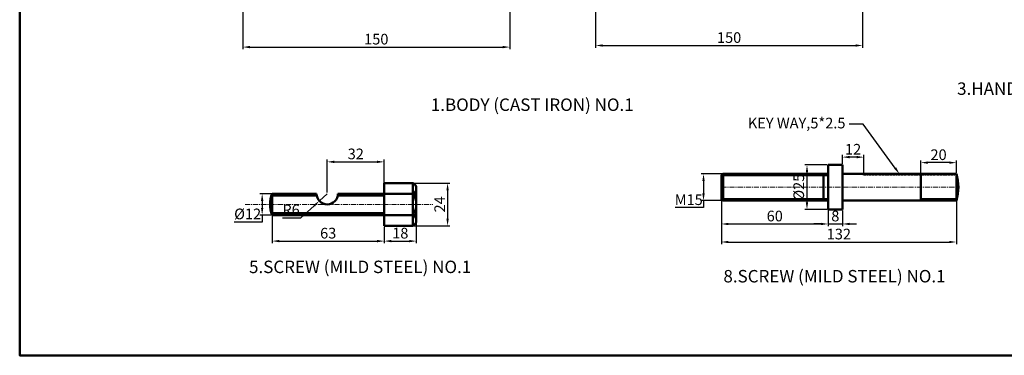
# Model space of a CAD drawing. Units: millimetres. Extents: x 177 to 1064, y 105 to 671.
# Tile 1 of 4: x 177 to 730, y 105 to 294. Entities that reach past the tile are written whole.
import ezdxf
from ezdxf import colors
from ezdxf.entities.mleader import LeaderData, LeaderLine
from ezdxf.math import Vec2, Vec3

# ---------------------------------------------------------------- set-up
doc = ezdxf.new("R2010")
doc.units = ezdxf.units.MM
doc.header["$LTSCALE"] = 0.3
doc.linetypes.add('CENTER', pattern=[50.8, 31.75, -6.35, 6.35, -6.35])
doc.linetypes.add('HIDDEN', pattern=[9.525, 6.35, -3.175])
for name, color, linetype, lineweight in [('M-CNTR', 1, 'CENTER', 18), ('M-DIMS', 2, 'Continuous', 25), ('M-HIDN', 6, 'HIDDEN', 25), ('M-OUTL', 7, 'Continuous', 50), ('M-TEXT', 3, 'Continuous', 25)]:
    doc.layers.add(name, color=color, linetype=linetype, lineweight=lineweight)
doc.styles.get("Standard").update_dxf_attribs({"font": 'arial.ttf'})
doc.dimstyles.new('ISO-25', dxfattribs={"dimtxt": 6, "dimasz": 4, "dimexe": 1.25, "dimexo": 0.625, "dimtad": 1, "dimtoh": 1, "dimtxsty": 'Standard', "dimcen": 2.5, "dimadec": 0, "dimazin": 0, "dimtfac": 1, "dimtmove": 0, "dimatfit": 3, "dimfxl": 1, "dimarcsym": 0})

# ---------------------------------------------------------------- blocks, each defined once
blk = doc.blocks.new('*D1')
at = {"layer": 'Defpoints', "color": 0, "ltscale": 0.2, "transparency": 16777216}
for p in [(302.04, 325.34), (452.04, 325.34), (452.04, 278.47)]:
    blk.add_point(p, dxfattribs=at)
at = {"layer": 'M-DIMS', "color": 0, "lineweight": -2, "ltscale": 0.2, "transparency": 16777216}
for p, q in [((302.04, 324.72), (302.04, 277.22)), ((452.04, 324.72), (452.04, 277.22)), ((306.04, 278.47), (448.04, 278.47))]:
    blk.add_line(p, q, dxfattribs=at)
at = {"layer": 'M-DIMS', "color": 0, "ltscale": 0.2, "transparency": 16777216}
for points in [[(306.04, 279.14), (306.04, 277.81), (302.04, 278.47)], [(448.04, 279.14), (448.04, 277.81), (452.04, 278.47)]]:
    blk.add_solid(points, dxfattribs=at)
at = {"layer": 'M-DIMS', "color": 0, "ltscale": 0.2, "transparency": 16777216, "insert": (377.04, 282.16), "char_height": 6, "attachment_point": 5}
blk.add_mtext('150', dxfattribs=at)
blk = doc.blocks.new('*D17')
at = {"layer": 'Defpoints', "color": 0, "ltscale": 0.2, "transparency": 16777216}
for p in [(500.2, 315.34), (650.2, 315.34), (650.2, 279.36)]:
    blk.add_point(p, dxfattribs=at)
at = {"layer": 'M-DIMS', "color": 0, "lineweight": -2, "ltscale": 0.2, "transparency": 16777216}
for p, q in [((500.2, 314.72), (500.2, 278.11)), ((650.2, 314.72), (650.2, 278.11)), ((504.2, 279.36), (646.2, 279.36))]:
    blk.add_line(p, q, dxfattribs=at)
at = {"layer": 'M-DIMS', "color": 0, "ltscale": 0.2, "transparency": 16777216}
for points in [[(504.2, 280.03), (504.2, 278.7), (500.2, 279.36)], [(646.2, 280.03), (646.2, 278.7), (650.2, 279.36)]]:
    blk.add_solid(points, dxfattribs=at)
at = {"layer": 'M-DIMS', "color": 0, "ltscale": 0.2, "transparency": 16777216, "insert": (575.2, 283.05), "char_height": 6, "attachment_point": 5}
blk.add_mtext('150', dxfattribs=at)
blk = doc.blocks.new('*D33')
at = {"layer": 'Defpoints', "color": 0, "ltscale": 0.3, "transparency": 16777216}
for p in [(381.52, 213.92), (349.52, 196), (381.52, 196)]:
    blk.add_point(p, dxfattribs=at)
at = {"layer": 'M-DIMS', "color": 0, "lineweight": -2, "ltscale": 0.3, "transparency": 16777216}
for p, q in [((349.52, 196.63), (349.52, 215.17)), ((353.52, 213.92), (377.52, 213.92)), ((381.52, 196.63), (381.52, 215.17))]:
    blk.add_line(p, q, dxfattribs=at)
at = {"layer": 'M-DIMS', "color": 0, "ltscale": 0.3, "transparency": 16777216}
for points in [[(353.52, 214.59), (353.52, 213.25), (349.52, 213.92)], [(377.52, 214.59), (377.52, 213.25), (381.52, 213.92)]]:
    blk.add_solid(points, dxfattribs=at)
at = {"layer": 'M-DIMS', "color": 0, "ltscale": 0.3, "transparency": 16777216, "insert": (365.52, 217.61), "char_height": 6, "attachment_point": 5}
blk.add_mtext('32', dxfattribs=at)
blk = doc.blocks.new('*D34')
at = {"layer": 'Defpoints', "color": 0, "ltscale": 0.3, "transparency": 16777216}
for p in [(318.52, 184), (381.52, 178), (381.52, 169.36)]:
    blk.add_point(p, dxfattribs=at)
at = {"layer": 'M-DIMS', "color": 0, "lineweight": -2, "ltscale": 0.3, "transparency": 16777216}
for p, q in [((318.52, 183.38), (318.52, 168.11)), ((381.52, 177.38), (381.52, 168.11)), ((322.52, 169.36), (377.52, 169.36))]:
    blk.add_line(p, q, dxfattribs=at)
at = {"layer": 'M-DIMS', "color": 0, "ltscale": 0.3, "transparency": 16777216}
for points in [[(322.52, 170.03), (322.52, 168.69), (318.52, 169.36)], [(377.52, 170.03), (377.52, 168.69), (381.52, 169.36)]]:
    blk.add_solid(points, dxfattribs=at)
at = {"layer": 'M-DIMS', "color": 0, "ltscale": 0.3, "transparency": 16777216, "insert": (350.02, 173.05), "char_height": 6, "attachment_point": 5}
blk.add_mtext('63', dxfattribs=at)
blk = doc.blocks.new('*D35')
at = {"layer": 'Defpoints', "color": 0, "ltscale": 0.3, "transparency": 16777216}
for p in [(331.02, 196), (312.94, 184), (331.02, 184)]:
    blk.add_point(p, dxfattribs=at)
at = {"layer": 'M-DIMS', "color": 0, "lineweight": -2, "ltscale": 0.3, "transparency": 16777216}
for p, q in [((330.4, 196), (311.69, 196)), ((312.94, 192), (312.94, 188)), ((330.4, 184), (311.69, 184)), ((312.94, 184), (312.94, 180)), ((312.94, 180), (297.26, 180))]:
    blk.add_line(p, q, dxfattribs=at)
at = {"layer": 'M-DIMS', "color": 0, "ltscale": 0.3, "transparency": 16777216}
for points in [[(312.28, 192), (313.61, 192), (312.94, 196)], [(312.28, 188), (313.61, 188), (312.94, 184)]]:
    blk.add_solid(points, dxfattribs=at)
at = {"layer": 'M-DIMS', "color": 0, "ltscale": 0.3, "transparency": 16777216, "insert": (304.79, 183.86), "char_height": 6, "attachment_point": 5}
blk.add_mtext('%%C12', dxfattribs=at)
blk = doc.blocks.new('*D36')
at = {"layer": 'Defpoints', "color": 0, "ltscale": 0.3, "transparency": 16777216}
for p in [(399.52, 184), (381.52, 178), (399.52, 169.36)]:
    blk.add_point(p, dxfattribs=at)
at = {"layer": 'M-DIMS', "color": 0, "lineweight": -2, "ltscale": 0.3, "transparency": 16777216}
for p, q in [((399.52, 183.38), (399.52, 168.11)), ((381.52, 177.38), (381.52, 168.11)), ((385.52, 169.36), (395.52, 169.36))]:
    blk.add_line(p, q, dxfattribs=at)
at = {"layer": 'M-DIMS', "color": 0, "ltscale": 0.3, "transparency": 16777216}
for points in [[(385.52, 170.03), (385.52, 168.69), (381.52, 169.36)], [(395.52, 170.03), (395.52, 168.69), (399.52, 169.36)]]:
    blk.add_solid(points, dxfattribs=at)
at = {"layer": 'M-DIMS', "color": 0, "ltscale": 0.3, "transparency": 16777216, "insert": (390.52, 173.05), "char_height": 6, "attachment_point": 5}
blk.add_mtext('18', dxfattribs=at)
blk = doc.blocks.new('*D37')
at = {"layer": 'Defpoints', "color": 0, "ltscale": 0.3, "transparency": 16777216}
for p in [(570.84, 199.67), (630.84, 199.67), (630.84, 178.99)]:
    blk.add_point(p, dxfattribs=at)
at = {"layer": 'M-DIMS', "color": 0, "lineweight": -2, "ltscale": 0.3, "transparency": 16777216}
for p, q in [((570.84, 199.04), (570.84, 177.74)), ((630.84, 199.04), (630.84, 177.74)), ((574.84, 178.99), (626.84, 178.99))]:
    blk.add_line(p, q, dxfattribs=at)
at = {"layer": 'M-DIMS', "color": 0, "ltscale": 0.3, "transparency": 16777216}
for points in [[(574.84, 179.65), (574.84, 178.32), (570.84, 178.99)], [(626.84, 179.65), (626.84, 178.32), (630.84, 178.99)]]:
    blk.add_solid(points, dxfattribs=at)
at = {"layer": 'M-DIMS', "color": 0, "ltscale": 0.3, "transparency": 16777216, "insert": (600.84, 182.67), "char_height": 6, "attachment_point": 5}
blk.add_mtext('60', dxfattribs=at)
blk = doc.blocks.new('*D38')
at = {"layer": 'Defpoints', "color": 0, "ltscale": 0.3, "transparency": 16777216}
for p in [(578.45, 207.17), (560.82, 192.17), (578.45, 192.17)]:
    blk.add_point(p, dxfattribs=at)
at = {"layer": 'M-DIMS', "color": 0, "lineweight": -2, "ltscale": 0.3, "transparency": 16777216}
for p, q in [((577.83, 207.17), (559.57, 207.17)), ((560.82, 203.17), (560.82, 196.17)), ((560.82, 188.17), (544.85, 188.17)), ((577.83, 192.17), (559.57, 192.17)), ((560.82, 192.17), (560.82, 188.17))]:
    blk.add_line(p, q, dxfattribs=at)
at = {"layer": 'M-DIMS', "color": 0, "ltscale": 0.3, "transparency": 16777216}
for points in [[(560.15, 203.17), (561.49, 203.17), (560.82, 207.17)], [(560.15, 196.17), (561.49, 196.17), (560.82, 192.17)]]:
    blk.add_solid(points, dxfattribs=at)
at = {"layer": 'M-DIMS', "color": 0, "ltscale": 0.3, "transparency": 16777216, "insert": (552.52, 191.86), "char_height": 6, "attachment_point": 5}
blk.add_mtext('M15', dxfattribs=at)
blk = doc.blocks.new('*D39')
at = {"layer": 'Defpoints', "color": 0, "ltscale": 0.3, "transparency": 16777216}
for p in [(630.84, 212.17), (618.94, 187.17), (630.84, 187.17)]:
    blk.add_point(p, dxfattribs=at)
at = {"layer": 'M-DIMS', "color": 0, "lineweight": -2, "ltscale": 0.3, "transparency": 16777216}
for p, q in [((630.21, 212.17), (617.69, 212.17)), ((618.94, 208.17), (618.94, 191.17)), ((630.21, 187.17), (617.69, 187.17))]:
    blk.add_line(p, q, dxfattribs=at)
at = {"layer": 'M-DIMS', "color": 0, "ltscale": 0.3, "transparency": 16777216}
for points in [[(618.27, 208.17), (619.6, 208.17), (618.94, 212.17)], [(618.27, 191.17), (619.6, 191.17), (618.94, 187.17)]]:
    blk.add_solid(points, dxfattribs=at)
at = {"layer": 'M-DIMS', "color": 0, "ltscale": 0.3, "transparency": 16777216, "insert": (615.08, 199.67), "char_height": 6, "attachment_point": 5, "rotation": 90}
blk.add_mtext('%%C25', dxfattribs=at)
blk = doc.blocks.new('*D40')
at = {"layer": 'Defpoints', "color": 0, "ltscale": 0.3, "transparency": 16777216}
for p in [(630.84, 187.17), (638.84, 187.17), (638.84, 178.99)]:
    blk.add_point(p, dxfattribs=at)
at = {"layer": 'M-DIMS', "color": 0, "lineweight": -2, "ltscale": 0.3, "transparency": 16777216}
for p, q in [((630.84, 186.54), (630.84, 177.74)), ((638.84, 186.54), (638.84, 177.74)), ((626.84, 178.99), (622.84, 178.99)), ((630.84, 178.99), (638.84, 178.99)), ((642.84, 178.99), (646.84, 178.99))]:
    blk.add_line(p, q, dxfattribs=at)
at = {"layer": 'M-DIMS', "color": 0, "ltscale": 0.3, "transparency": 16777216}
for points in [[(626.84, 179.65), (626.84, 178.32), (630.84, 178.99)], [(642.84, 179.65), (642.84, 178.32), (638.84, 178.99)]]:
    blk.add_solid(points, dxfattribs=at)
at = {"layer": 'M-DIMS', "color": 0, "ltscale": 0.3, "transparency": 16777216, "insert": (634.84, 182.67), "char_height": 6, "attachment_point": 5}
blk.add_mtext('8', dxfattribs=at)
blk = doc.blocks.new('*D41')
at = {"layer": 'Defpoints', "color": 0, "ltscale": 0.3, "transparency": 16777216}
for p in [(702.84, 199.67), (570.84, 188.39), (702.84, 168.85)]:
    blk.add_point(p, dxfattribs=at)
at = {"layer": 'M-DIMS', "color": 0, "lineweight": -2, "ltscale": 0.3, "transparency": 16777216}
for p, q in [((702.84, 199.04), (702.84, 167.6)), ((570.84, 187.76), (570.84, 167.6)), ((574.84, 168.85), (698.84, 168.85))]:
    blk.add_line(p, q, dxfattribs=at)
at = {"layer": 'M-DIMS', "color": 0, "ltscale": 0.3, "transparency": 16777216}
for points in [[(574.84, 169.51), (574.84, 168.18), (570.84, 168.85)], [(698.84, 169.51), (698.84, 168.18), (702.84, 168.85)]]:
    blk.add_solid(points, dxfattribs=at)
at = {"layer": 'M-DIMS', "color": 0, "ltscale": 0.3, "transparency": 16777216, "insert": (636.84, 172.54), "char_height": 6, "attachment_point": 5}
blk.add_mtext('132', dxfattribs=at)
blk = doc.blocks.new('*D42')
at = {"layer": 'Defpoints', "color": 0, "ltscale": 0.3, "transparency": 16777216}
for p in [(682.84, 213.48), (682.84, 207.17), (702.84, 207.17)]:
    blk.add_point(p, dxfattribs=at)
at = {"layer": 'M-DIMS', "color": 0, "lineweight": -2, "ltscale": 0.3, "transparency": 16777216}
for p, q in [((682.84, 207.79), (682.84, 214.73)), ((698.84, 213.48), (686.84, 213.48)), ((702.84, 207.79), (702.84, 214.73))]:
    blk.add_line(p, q, dxfattribs=at)
at = {"layer": 'M-DIMS', "color": 0, "ltscale": 0.3, "transparency": 16777216}
for points in [[(686.84, 214.15), (686.84, 212.82), (682.84, 213.48)], [(698.84, 214.15), (698.84, 212.82), (702.84, 213.48)]]:
    blk.add_solid(points, dxfattribs=at)
at = {"layer": 'M-DIMS', "color": 0, "ltscale": 0.3, "transparency": 16777216, "insert": (692.84, 217.17), "char_height": 6, "attachment_point": 5}
blk.add_mtext('20', dxfattribs=at)
blk = doc.blocks.new('*D43')
at = {"layer": 'Defpoints', "color": 0, "ltscale": 0.3, "transparency": 16777216}
for p in [(638.84, 216.59), (638.84, 212.17), (650.84, 207.17)]:
    blk.add_point(p, dxfattribs=at)
at = {"layer": 'M-DIMS', "color": 0, "lineweight": -2, "ltscale": 0.3, "transparency": 16777216}
for p, q in [((638.84, 212.79), (638.84, 217.84)), ((646.84, 216.59), (642.84, 216.59)), ((650.84, 207.79), (650.84, 217.84))]:
    blk.add_line(p, q, dxfattribs=at)
at = {"layer": 'M-DIMS', "color": 0, "ltscale": 0.3, "transparency": 16777216}
for points in [[(642.84, 217.26), (642.84, 215.92), (638.84, 216.59)], [(646.84, 217.26), (646.84, 215.92), (650.84, 216.59)]]:
    blk.add_solid(points, dxfattribs=at)
at = {"layer": 'M-DIMS', "color": 0, "ltscale": 0.3, "transparency": 16777216, "insert": (644.84, 220.23), "char_height": 6, "attachment_point": 5}
blk.add_mtext('12', dxfattribs=at)
blk = doc.blocks.new('*D66')
at = {"layer": 'Defpoints', "color": 0, "ltscale": 0.3, "transparency": 16777216}
for p in [(381.52, 202), (381.52, 178), (417.08, 178)]:
    blk.add_point(p, dxfattribs=at)
at = {"layer": 'M-DIMS', "color": 0, "lineweight": -2, "ltscale": 0.3, "transparency": 16777216}
for p, q in [((382.15, 202), (418.33, 202)), ((417.08, 198), (417.08, 182)), ((382.15, 178), (418.33, 178))]:
    blk.add_line(p, q, dxfattribs=at)
at = {"layer": 'M-DIMS', "color": 0, "ltscale": 0.3, "transparency": 16777216}
for points in [[(416.41, 198), (417.74, 198), (417.08, 202)], [(416.41, 182), (417.74, 182), (417.08, 178)]]:
    blk.add_solid(points, dxfattribs=at)
at = {"layer": 'M-DIMS', "color": 0, "ltscale": 0.3, "transparency": 16777216, "insert": (413.44, 190), "char_height": 6, "attachment_point": 5, "rotation": 90}
blk.add_mtext('24', dxfattribs=at)
blk = doc.blocks.new('*D73')
at = {"layer": 'Defpoints', "color": 0, "ltscale": 0.3, "transparency": 16777216}
for p in [(349.52, 196), (345.08, 191.96)]:
    blk.add_point(p, dxfattribs=at)
at = {"layer": 'M-DIMS', "color": 0, "lineweight": -2, "ltscale": 0.3, "transparency": 16777216}
for p, q in [((349.52, 196), (345.08, 191.96)), ((334.63, 182.46), (342.12, 189.27)), ((324.33, 182.46), (334.63, 182.46))]:
    blk.add_line(p, q, dxfattribs=at)
at = {"layer": 'M-DIMS', "color": 0, "ltscale": 0.3, "transparency": 16777216}
blk.add_solid([(341.67, 189.77), (342.57, 188.78), (345.08, 191.96)], dxfattribs=at)
at = {"layer": 'M-DIMS', "color": 0, "ltscale": 0.3, "transparency": 16777216, "insert": (329.17, 186.15), "char_height": 6, "attachment_point": 5}
blk.add_mtext('R6', dxfattribs=at)

msp = doc.modelspace()

# ---------------------------------------------------------------- linework, layer by layer
at = {"layer": 'M-CNTR', "ltscale": 0.3}
for p, q in [((570.8359, 199.6679), (703.9824, 199.6679)), ((303.3169, 190.0007), (408.7771, 190.0007))]:
    msp.add_line(p, q, dxfattribs=at)
at = {"layer": 'M-HIDN', "ltscale": 0.3}
msp.add_line((702.8359, 206.4179), (650.8359, 206.4179), dxfattribs=at)
at = {"layer": 'M-OUTL', "ltscale": 0.3}
for p, q in [((630.8359, 212.1679), (630.8359, 187.1679)), ((638.8359, 212.1679), (630.8359, 212.1679)), ((638.8359, 187.1679), (638.8359, 212.1679)), ((571.8359, 207.1679), (570.8359, 206.5906)), ((570.8359, 206.5906), (570.8359, 192.7453)), ((630.8359, 207.1679), (571.8359, 207.1679)), ((571.8359, 207.1679), (571.8359, 192.1679)), ((630.8359, 206.4179), (571.8359, 206.4179)), ((628.2094, 207.1679), (628.2094, 192.1679)), ((630.8359, 192.1679), (630.8359, 207.1679)), ((702.8359, 207.1679), (638.8359, 207.1679)), ((650.8359, 206.4179), (650.8359, 207.1679)), ((682.8359, 192.1679), (682.8359, 207.1679)), ((702.8359, 192.1679), (702.8359, 207.1679)), ((381.52, 178.0007), (381.52, 202.0007)), ((381.52, 202.0007), (397.52, 202.0007)), ((397.52, 202.0007), (397.52, 178.0007)), ((399.52, 199.2197), (399.52, 180.8116)), ((318.52, 196.0007), (343.52, 196.0007)), ((318.52, 196.0007), (318.52, 184.0007)), ((318.52, 195.0007), (343.6039, 195.0007)), ((355.4361, 195.0007), (381.52, 195.0007)), ((355.52, 196.0007), (399.52, 196.0007)), ((571.8359, 192.1679), (570.8359, 192.7453)), ((571.8359, 192.9179), (630.8359, 192.9179)), ((571.8359, 192.1679), (630.8359, 192.1679)), ((702.8359, 192.1679), (638.8359, 192.1679)), ((702.8359, 192.9179), (682.8359, 192.9179)), ((318.52, 185.0007), (381.52, 185.0007)), ((318.52, 184.0007), (399.52, 184.0007)), ((630.8359, 187.1679), (638.8359, 187.1679)), ((397.52, 178.0007), (381.52, 178.0007))]:
    msp.add_line(p, q, dxfattribs=at)
msp.add_lwpolyline([(176.7558, 671.1865), (1063.6064, 671.1865), (1063.6064, 105.1095), (176.7558, 105.1095)], close=True, dxfattribs=at)
for centre, radius, start, end in [((678.8774, 199.6679), 25.105, 342.61771, 17.38229), ((396.282, 199.0007), 3.2454, 292.424309, 67.575691), ((333.763, 190.0007), 16.3813, 158.514213, 201.485787), ((349.52, 196.0007), 6, 180, 0), ((389.52, 190.0007), 10, 323.130102, 36.869898), ((396.2789, 181.0007), 3.2466, 292.474338, 67.525662)]:
    msp.add_arc(centre, radius, start, end, dxfattribs=at)

# ---------------------------------------------------------------- texts
at = {"layer": 'M-TEXT', "ltscale": 0.3, "char_height": 7, "attachment_point": 1}
for s, width, insert in [('\\pxqc;3.HAND WHEEL (CAST STEEL) NO.1', 180.935096, (689.8312, 258.6014)), ('\\pxqc;1.BODY (CAST IRON) NO.1', 180.935096, (374.1667, 249.5619)), ('\\pxqc;5.SCREW (MILD STEEL) NO.1', 193.296097, (271.3193, 158.3658)), ('\\pxqc;8.SCREW (MILD STEEL) NO.1', 180.935096, (543.9199, 153.1132))]:
    msp.add_mtext_dynamic_manual_height_columns(s, width=width, gutter_width=12.5, heights=[0], dxfattribs=dict(at, insert=insert))

# ---------------------------------------------------------------- dimensions: what is measured, and where the dimension line sits
at = {"layer": 'M-DIMS', "ltscale": 0.2}
for base, p1, p2, picture, middle in [((452.0432, 278.4731), (302.0432, 325.3423), (452.0432, 325.3423), '*D1', (377.0432, 282.1615)), ((650.1968, 279.3639), (500.1968, 315.3423), (650.1968, 315.3423), '*D17', (575.1968, 283.0523))]:
    dim = msp.add_linear_dim(base=base, p1=p1, p2=p2, dimstyle='ISO-25', override={"dimclrd": 0, "dimclre": 0, "dimclrt": 0}, dxfattribs=at)
    dim.commit()
    dim.dimension.update_dxf_attribs({"geometry": picture, "text_midpoint": middle})
at = {"layer": 'M-DIMS', "ltscale": 0.3}
for base, p1, p2, picture, middle in [((381.52, 213.9203), (349.52, 196.0007), (381.52, 196.0007), '*D33', (365.52, 217.6108)), ((638.8359, 216.5897), (650.8359, 207.1679), (638.8359, 212.1679), '*D43', (644.8359, 220.2269)), ((682.8359, 213.4839), (702.8359, 207.1679), (682.8359, 207.1679), '*D42', (692.8359, 217.1723)), ((630.8359, 178.9858), (570.8359, 199.6679), (630.8359, 199.6679), '*D37', (600.8359, 182.6742)), ((702.8359, 168.848), (570.8359, 188.3894), (702.8359, 199.6679), '*D41', (636.8359, 172.5385)), ((381.52, 169.3609), (318.52, 184.0007), (381.52, 178.0007), '*D34', (350.02, 173.0513)), ((638.8359, 178.9858), (630.8359, 187.1679), (638.8359, 187.1679), '*D40', (634.8359, 182.6742))]:
    dim = msp.add_linear_dim(base=base, p1=p1, p2=p2, dimstyle='ISO-25', override={"dimclrd": 0, "dimclre": 0, "dimclrt": 0}, dxfattribs=at)
    dim.commit()
    dim.dimension.update_dxf_attribs({"geometry": picture, "text_midpoint": middle})
for base, p1, p2, text, picture, middle in [((618.9353, 187.1679), (630.8359, 212.1679), (630.8359, 187.1679), '%%C<>', '*D39', (615.0791, 199.6679)), ((560.8196, 192.1679), (578.4518, 207.1679), (578.4518, 192.1679), 'M<>', '*D38', (552.5207, 191.8564)), ((312.9429, 184.0007), (331.02, 196.0007), (331.02, 184.0007), '%%C<>', '*D35', (304.7872, 183.8569))]:
    dim = msp.add_linear_dim(base=base, p1=p1, p2=p2, angle=90, text=text, dimstyle='ISO-25', override={"dimclrd": 0, "dimclre": 0, "dimclrt": 0}, dxfattribs=at)
    dim.commit()
    dim.dimension.update_dxf_attribs({"geometry": picture, "text_midpoint": middle})
dim = msp.add_linear_dim(base=(417.0771, 178.0007), p1=(381.52, 202.0007), p2=(381.52, 178.0007), angle=90, dimstyle='ISO-25', override={"dimdec": 0, "dimlfac": 1, "dimrnd": 0, "dimzin": 0, "dimdsep": 46, "dimlunit": 2}, dxfattribs=at)
dim.commit()
dim.dimension.update_dxf_attribs({"geometry": '*D66', "text_midpoint": (413.4398, 190.0007)})
dim = msp.add_radius_dim(center=(349.52, 196.0007), mpoint=(345.0807, 191.9643), dimstyle='ISO-25', override={"dimdec": 0, "dimlfac": 1, "dimrnd": 0, "dimzin": 0, "dimdsep": 46, "dimlunit": 2}, dxfattribs=at)
dim.commit()
dim.dimension.update_dxf_attribs({"geometry": '*D73', "text_midpoint": (329.1678, 186.1491)})
dim = msp.add_linear_dim(base=(399.52, 169.3609), p1=(381.52, 178.0007), p2=(399.52, 184.0007), dimstyle='ISO-25', override={"dimclrd": 0, "dimclre": 0, "dimclrt": 0}, dxfattribs=at)
dim.commit()
dim.dimension.update_dxf_attribs({"geometry": '*D36', "text_midpoint": (390.52, 169.3609), "dimtype": 160})

# ---------------------------------------------------------------- leaders
ml = msp.add_multileader_mtext('Standard', dxfattribs=at)
ml.set_content('KEY WAY,5*2.5', color=256)
ml.set_leader_properties()
ml.build(insert=Vec2(0, 0))
ctx = ml.context
ctx.base_point, ctx.char_height, ctx.plane_origin = Vec3(579.3975, 235.1527), 6, Vec3(670.8359, 207.1679)
ctx.text_align_type = 2
notes = []
notes.append((ctx, [(0, (1, 1, 0), (650.5462, 235.1527), (-1, 0), 8, [(0, [(670.8359, 207.1679)], 0, [])])]))
ctx.mtext.insert, ctx.mtext.alignment, ctx.mtext.flow_direction = Vec3(640.5462, 238.7462), 3, 5
for ctx, leaders in notes:
    for number, flags, end, landing, length, lines in leaders:
        leader = LeaderData()
        leader.index, (leader.has_last_leader_line, leader.has_dogleg_vector, leader.attachment_direction) = number, flags
        leader.last_leader_point, leader.dogleg_vector, leader.dogleg_length = Vec3(end), Vec3(landing), length
        for number, points, colour, breaks in lines:
            line = LeaderLine()
            line.index, line.vertices, line.color, line.breaks = number, Vec3.list(points), colors.encode_raw_color(colour), breaks
            leader.lines.append(line)
        ctx.leaders.append(leader)

doc.saveas('drawing.dxf')
